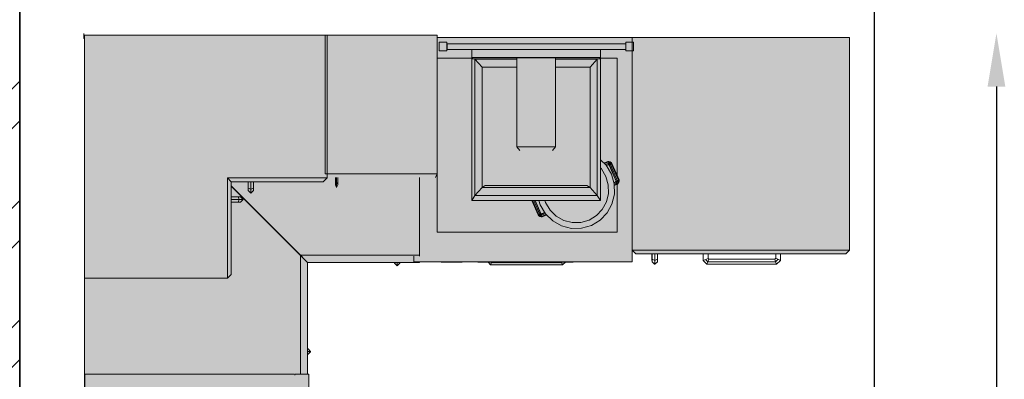
# Model space of a CAD drawing. Units: inches. Extents: x 3614 to 4242, y 2406 to 3033.
# Tile 5 of 10: x 3697 to 3808, y 2896 to 2936. Entities that reach past the tile are written whole.
import ezdxf

# ---------------------------------------------------------------- set-up
doc = ezdxf.new("R2010")
doc.units = ezdxf.units.IN
for name, color, linetype, lineweight in [('A-ANNO-DIMS', 2, 'Continuous', 18), ('A-FLOR-FIXT', 9, 'Continuous', 18), ('A-WALL', 7, 'Continuous', 35), ('A-WALL-PATT', 252, 'Continuous', 13)]:
    doc.layers.add(name, color=color, linetype=linetype, lineweight=lineweight)
doc.layers.add('hatch', color=254, linetype='Continuous')
doc.styles.get("Standard").update_dxf_attribs({"font": 'arial.ttf'})
doc.dimstyles.get("Standard").update_dxf_attribs({"dimtxt": 6, "dimasz": 6, "dimexe": 0.18, "dimexo": 0.0625, "dimgap": 0.09, "dimtad": 0, "dimtih": 1, "dimtoh": 1, "dimdec": 4, "dimzin": 0, "dimdsep": 46, "dimlunit": 4, "dimtxsty": 'Standard', "dimcen": 0.09, "dimse1": 1, "dimse2": 1, "dimadec": 0, "dimazin": 0, "dimtfac": 1, "dimtdec": 4, "dimtofl": 0, "dimtmove": 0, "dimatfit": 3, "dimfxl": 1, "dimtolj": 1, "dimtzin": 0, "dimarcsym": 0})

# ---------------------------------------------------------------- blocks, each defined once
blk = doc.blocks.new('kithen1')
at = {"layer": 'hatch'}
blk.add_hatch(color=256, dxfattribs=at).paths.add_polyline_path([(-2799.7, -8.3), (-2273.3, -8.3), (-2273.3, -1.7), (-2257.5, -1.7), (-2257.5, -1.1), (-1023.7, -1.1), (-1023.7, 0), (0, 0), (0, -0.3), (0.3, -0.3), (0.3, -1009.9), (-6.1, -1009.9), (-6.1, -2189.3), (-615.8, -2189.3), (-626.5, -2178.9), (-626.5, -1578.2), (-615.8, -1567.8), (-649.5, -1567.8), (-649.5, -1399.1), (-650.3, -1399.1), (-650.3, -1376.8), (-657.9, -1368.5), (-657.8, -1162.4), (-650.3, -1155.1), (-650.3, -1126.4), (-649.5, -1126.4), (-649.5, -1081.1), (-650.3, -1081.1), (-650.3, -1021.1), (-649.5, -1021.1), (-649.5, -959.1), (-651, -959.1), (-650.7, -903), (-653.5, -903), (-660.6, -895.5), (-660.5, -894.6), (-653.5, -887.1), (-651, -887.1), (-651, -638.7), (-651.2, -638.5), (-898.3, -638.5), (-898.3, -640.4), (-905.9, -647.4), (-906.8, -647.4), (-914.3, -640.4), (-914.3, -638.5), (-971.4, -638.5), (-971.4, -642.6), (-1016.2, -642.6), (-1016.2, -643.9), (-1023.8, -650.9), (-1024.7, -650.9), (-1032.2, -643.9), (-1032.2, -642.6), (-1179.7, -642.6), (-1188.8, -650.9), (-1395.6, -650.9), (-1403.7, -642.6), (-1813.5, -642.6), (-1822.6, -650.9), (-2029.4, -650.9), (-2037.5, -642.6), (-2257.5, -642.6), (-2257.5, -618.1), (-2261.3, -618.1), (-2271.7, -628.7), (-2458, -628.7), (-2727.7, -628.7), (-2727.7, -651.1), (-2735, -658.1), (-2735.9, -658), (-2743.2, -651.1), (-2743.2, -628.7), (-2789.4, -628.7), (-2799.7, -618.1)])
at = {"color": 0}
for p, q in [((0, 0), (-1023.7, 0)), ((-696.5, 0), (-696.5, -409.2)), ((-8.6, 1.9), (-10.5, 0)), ((-10.1, 0), (-8.2, 1.9)), ((-8.2, 1.9), (-8.3, 1.8)), ((-8.3, 1.9), (-8.3, 0)), ((5.4, 1.8), (-8.3, 1.8)), ((0, 0), (0, -694.7)), ((0, -0.3), (0, 0)), ((-2261.3, -8.3), (-2799.7, -8.3)), ((-2799.7, -8.3), (-2799.7, -618.1)), ((-2273.3, -1.9), (-2273.9, -1.9)), ((-2273.9, -1.9), (-2273.9, -8.3)), ((-2261.3, -1.7), (-2273.3, -1.7)), ((-2273.3, -1.7), (-2273.3, -8.3)), ((-2261.3, -601.6), (-2261.3, -1.7)), ((-2261.3, -618.1), (-2261.3, -8.3)), ((-2261, -8.5), (-2261.3, -8.5)), ((-971.4, -1.1), (-2257.5, -1.1)), ((-2257.5, -1.1), (-2257.5, -642.6)), ((-1023.7, -22.5), (-2210.1, -22.5)), ((-2210.1, -22.5), (-2210.1, -589.1)), ((-1023.7, -589.1), (-1023.7, -22.5)), ((-971.4, -1.1), (-971.4, -600.9)), ((0.3, -0.3), (0, -0.3)), ((0.3, -671.1), (0.3, -0.3)), ((-2257.5, -51.5), (-2261.3, -51.5)), ((-2261.3, -51.5), (-2261.3, -536.3)), ((-2183.7, -48.8), (-1056.9, -48.9)), ((-2169.4, -62.7), (-2183.7, -48.8)), ((-2183.7, -48.8), (-2183.7, -565)), ((-1056.9, -48.9), (-1071, -63.6)), ((-1056.9, -48.9), (-1056.9, -565)), ((-2169.7, -550.2), (-2169.4, -62.7)), ((-1071, -63.6), (-2169.4, -62.7)), ((-2103.6, -76.6), (-2136.6, -97.6)), ((-2135.1, -98.9), (-2102.3, -78.1)), ((-2100.1, -80.6), (-2132.5, -101.2)), ((-2057.7, -68.5), (-2103.6, -76.6)), ((-2102.3, -78.1), (-2056.8, -70)), ((-2100.1, -80.6), (-2102.3, -78.1)), ((-2055, -72.6), (-2100.1, -80.6)), ((-2093.2, -88.3), (-2100.1, -80.6)), ((-2049.7, -80.6), (-2093.2, -88.3)), ((-1740.9, -68.5), (-2057.7, -68.5)), ((-2056.8, -70), (-1741.9, -70)), ((-1743.7, -72.6), (-2055, -72.6)), ((-1749, -80.6), (-2049.7, -80.6)), ((-1716.2, -84.8), (-1749, -80.6)), ((-1709.7, -76.9), (-1743.7, -72.6)), ((-1741.9, -70), (-1707.6, -74.4)), ((-1706.4, -72.9), (-1740.9, -68.5)), ((-1678, -91.5), (-1709.7, -76.9)), ((-1707.6, -74.4), (-1675.5, -89.1)), ((-1674.1, -87.7), (-1706.4, -72.9)), ((-1071, -550.2), (-1071, -63.6)), ((-2136.6, -97.6), (-2156.1, -126.2)), ((-2154.5, -127.3), (-2135.1, -98.9)), ((-2132.5, -101.2), (-2151.7, -129.3)), ((-2124.5, -108.2), (-2143, -135.3)), ((-2132.5, -101.2), (-2135.1, -98.9)), ((-2124.5, -108.2), (-2132.5, -101.2)), ((-2093.2, -88.3), (-2124.5, -108.2)), ((-1685.6, -98.8), (-1716.2, -84.8)), ((-1678, -91.5), (-1685.6, -98.8)), ((-1685.6, -98.8), (-1660.4, -125.8)), ((-1651.9, -119.5), (-1678, -91.5)), ((-1675.5, -89.1), (-1649.1, -117.4)), ((-1647.6, -116.2), (-1674.1, -87.7)), ((-1523.7, -95.6), (-1554, -114.9)), ((-1481.5, -88.1), (-1523.7, -95.6)), ((-1523.7, -95.6), (-1509.8, -111.1)), ((-1189.8, -88.1), (-1481.5, -88.1)), ((-1416.2, -122.1), (-1396, -106.6)), ((-1396, -106.6), (-1372.5, -96.9)), ((-1372.5, -96.9), (-1347.3, -93.6)), ((-1347.3, -93.6), (-1322, -96.9)), ((-1322, -96.9), (-1298.5, -106.6)), ((-1298.5, -106.6), (-1278.3, -122.1)), ((-1283.4, -118.2), (-1268.1, -102.9)), ((-1268.1, -102.9), (-1230.5, -92.9)), ((-1230.5, -92.9), (-1193, -102.9)), ((-1193, -102.9), (-1165.5, -130.3)), ((-1157.9, -92.2), (-1189.8, -88.1)), ((-1128.2, -105.8), (-1157.9, -92.2)), ((-1143.5, -120.5), (-1128.2, -105.8)), ((-1128.2, -105.8), (-1103.8, -132)), ((-2156.1, -126.2), (-2163.3, -163.2)), ((-2161.7, -164.1), (-2154.5, -127.3)), ((-2151.7, -129.3), (-2158.8, -165.7)), ((-2151.7, -129.3), (-2154.5, -127.3)), ((-2143, -135.3), (-2151.7, -129.3)), ((-2149.9, -170.5), (-2143, -135.3)), ((-1660.4, -125.8), (-1651.9, -119.5)), ((-1648.8, -170.4), (-1660.4, -125.8)), ((-1649.1, -117.4), (-1651.9, -119.5)), ((-1651.9, -119.5), (-1639.9, -165.7)), ((-1649.1, -117.4), (-1637, -164.1)), ((-1635.3, -163.2), (-1647.6, -116.2)), ((-1554, -114.9), (-1572, -141.2)), ((-1431.7, -142.2), (-1416.2, -122.1)), ((-1278.3, -122.1), (-1262.8, -142.2)), ((-1252, -130.7), (-1263.1, -141.8)), ((-1249.5, -134.9), (-1261, -146.4)), ((-1246.6, -139.9), (-1258.4, -151.7)), ((-1252, -130.7), (-1230.5, -124.9)), ((-1249.5, -134.9), (-1230.5, -129.8)), ((-1230.5, -135.6), (-1246.6, -139.9)), ((-1246.6, -139.9), (-1244.8, -143)), ((-1244.8, -143), (-1230.5, -139.2)), ((-1230.5, -124.9), (-1209.1, -130.7)), ((-1230.5, -129.8), (-1211.6, -134.9)), ((-1214.5, -139.9), (-1230.5, -135.6)), ((-1230.5, -135.6), (-1230.5, -139.2)), ((-1230.5, -139.2), (-1216.3, -143)), ((-1216.3, -143), (-1214.5, -139.9)), ((-1211.6, -134.9), (-1214.5, -139.9)), ((-1214.5, -139.9), (-1202.7, -151.7)), ((-1211.6, -134.9), (-1197.7, -148.8)), ((-1209.1, -130.7), (-1193.4, -146.3)), ((-1165.5, -130.3), (-1155.5, -167.7)), ((-1103.8, -132), (-1120.8, -144.8)), ((-1103.8, -132), (-1092.5, -175.3)), ((-2163.3, -163.2), (-2163.3, -447.5)), ((-2161.7, -446.6), (-2161.7, -164.1)), ((-2158.8, -165.7), (-2158.8, -445)), ((-1639.9, -165.7), (-1639.9, -445)), ((-1637, -164.1), (-1637, -446.6)), ((-1635.3, -447.4), (-1635.3, -163.2)), ((-1572, -141.2), (-1578.6, -175.3)), ((-1572, -141.2), (-1554.6, -153.3)), ((-1444.8, -190.8), (-1441.5, -165.7)), ((-1441.5, -165.7), (-1431.7, -142.2)), ((-1262.8, -142.2), (-1253, -165.7)), ((-1258.4, -151.7), (-1258.6, -152.3)), ((-1255.2, -153.5), (-1258.4, -151.7)), ((-1255.2, -153.5), (-1256.4, -157.6)), ((-1244.8, -143), (-1255.2, -153.5)), ((-1253, -165.7), (-1249.7, -190.8)), ((-1205.8, -153.5), (-1216.3, -143)), ((-1202.7, -151.7), (-1205.8, -153.5)), ((-1205.8, -153.5), (-1202, -167.7)), ((-1202, -167.7), (-1205.8, -181.9)), ((-1198.4, -167.7), (-1202.7, -151.7)), ((-1202.7, -183.7), (-1198.4, -167.7)), ((-1202, -167.7), (-1198.4, -167.7)), ((-1197.7, -148.8), (-1192.6, -167.7)), ((-1192.6, -167.7), (-1197.7, -186.6)), ((-1193.4, -146.3), (-1187.6, -167.7)), ((-1187.6, -167.7), (-1193.4, -189.1)), ((-1155.5, -167.7), (-1165.5, -205.1)), ((-2149.9, -440.2), (-2149.9, -170.5)), ((-1648.8, -440.2), (-1648.8, -170.4)), ((-1578.6, -175.3), (-1578.6, -437)), ((-1441.5, -216), (-1444.8, -190.8)), ((-1249.7, -190.8), (-1253, -216)), ((-1250.2, -186.9), (-1244.8, -192.3)), ((-1246.6, -195.5), (-1249.9, -192.2)), ((-1244.8, -192.3), (-1246.6, -195.5)), ((-1230.5, -199.7), (-1246.6, -195.5)), ((-1230.5, -196.1), (-1244.8, -192.3)), ((-1216.3, -192.3), (-1230.5, -196.1)), ((-1214.5, -195.5), (-1230.5, -199.7)), ((-1230.5, -196.1), (-1230.5, -199.7)), ((-1205.8, -181.9), (-1216.3, -192.3)), ((-1216.3, -192.3), (-1214.5, -195.5)), ((-1214.5, -195.5), (-1202.7, -183.7)), ((-1211.6, -200.5), (-1214.5, -195.5)), ((-1197.7, -186.6), (-1211.6, -200.5)), ((-1193.4, -189.1), (-1209.1, -204.7)), ((-1205.8, -181.9), (-1202.7, -183.7)), ((-1092.5, -175.3), (-1092.5, -437)), ((-1442, -212), (-1442.1, -213.6)), ((-1442.1, -213.6), (-1441.9, -216.3)), ((-1441.9, -216.3), (-1441.5, -218.2)), ((-1431.7, -239.4), (-1441.5, -216)), ((-1441.5, -218.2), (-1440.8, -218.9)), ((-1440.8, -218.9), (-1440.3, -218.9)), ((-1253, -216), (-1262.8, -239.4)), ((-1230.5, -210.4), (-1251.6, -204.8)), ((-1250.8, -199.1), (-1249.5, -200.5)), ((-1211.6, -200.5), (-1230.5, -205.5)), ((-1209.1, -204.7), (-1230.5, -210.4)), ((-1165.5, -205.1), (-1193, -232.5)), ((-1416.2, -259.6), (-1431.7, -239.4)), ((-1262.8, -239.4), (-1278.3, -259.6)), ((-1230.5, -242.5), (-1260.7, -234.4)), ((-1193, -232.5), (-1230.5, -242.5)), ((-1914.6, -272.1), (-1926.9, -292)), ((-1891.8, -266.6), (-1914.6, -272.1)), ((-1871.8, -278.8), (-1891.8, -266.6)), ((-1866.3, -301.6), (-1871.8, -278.8)), ((-1396, -275), (-1416.2, -259.6)), ((-1372.5, -284.8), (-1396, -275)), ((-1298.5, -275), (-1322, -284.8)), ((-1278.3, -259.6), (-1298.5, -275)), ((-1926.9, -292), (-1921.4, -314.8)), ((-1878.5, -321.5), (-1866.3, -301.6)), ((-1526.8, -324.6), (-1493.1, -302.1)), ((-1493.1, -302.2), (-1526.8, -324.6)), ((-1492.2, -304.2), (-1525.2, -326.2)), ((-1493.1, -302.1), (-1453.2, -294.2)), ((-1453.2, -294.3), (-1493.1, -302.2)), ((-1453.2, -296.5), (-1492.2, -304.2)), ((-1453.2, -294.2), (-1413.4, -302.1)), ((-1413.4, -302.2), (-1453.2, -294.3)), ((-1453.2, -294.3), (-1453.2, -296.5)), ((-1453.2, -296.5), (-1414.2, -304.2)), ((-1413.4, -302.1), (-1379.6, -324.6)), ((-1379.6, -324.6), (-1413.4, -302.2)), ((-1347.3, -288.1), (-1372.5, -284.8)), ((-1364, -321.4), (-1354.5, -287.1)), ((-1322, -284.8), (-1347.3, -288.1)), ((-1316.5, -282.5), (-1307.2, -290.8)), ((-1307.2, -290.8), (-1307.2, -321.4)), ((-1921.4, -314.8), (-1901.4, -327)), ((-1901.4, -327), (-1878.5, -321.5)), ((-1526.8, -324.6), (-1549.4, -358.3)), ((-1549.4, -358.3), (-1526.8, -324.6)), ((-1525.2, -326.2), (-1547.3, -359.2)), ((-1514.5, -337), (-1533.3, -365)), ((-1486.4, -318.2), (-1514.5, -337)), ((-1453.2, -311.7), (-1486.4, -318.2)), ((-1453.2, -311.7), (-1420.1, -318.2)), ((-1453.2, -338.2), (-1453.2, -311.7)), ((-1420.1, -318.2), (-1392, -337)), ((-1392, -337), (-1373.2, -365)), ((-1379.6, -324.6), (-1357, -358.3)), ((-1357, -358.3), (-1379.6, -324.6)), ((-1363.6, -324.3), (-1364, -321.4)), ((-1361.6, -328), (-1363.6, -324.3)), ((-1357.9, -330.6), (-1361.6, -328)), ((-1352.7, -331.6), (-1357.9, -330.6)), ((-1318.5, -331.6), (-1352.7, -331.6)), ((-1314.3, -331), (-1318.5, -331.6)), ((-1310.7, -329.1), (-1314.3, -331)), ((-1308.2, -326), (-1310.7, -329.1)), ((-1307.2, -321.4), (-1308.2, -326)), ((-1248.3, -343.1), (-1240.7, -330.6)), ((-1243.2, -344.9), (-1236.8, -334.2)), ((-1240.7, -330.6), (-1228.9, -321.9)), ((-1227.6, -324.8), (-1238.3, -332.8)), ((-1236.8, -334.2), (-1226.7, -326.8)), ((-1228.9, -321.9), (-1214.7, -318.4)), ((-1227.6, -324.8), (-1228.3, -323.3)), ((-1214.6, -321.6), (-1227.6, -324.8)), ((-1226.7, -326.8), (-1214.5, -323.7)), ((-1214.7, -318.4), (-1200.3, -320.6)), ((-1214.7, -319.9), (-1214.6, -321.6)), ((-1214.6, -321.6), (-1201.4, -323.6)), ((-1214.5, -323.7), (-1202.1, -325.6)), ((-1202.1, -325.6), (-1191.3, -332)), ((-1201.4, -323.6), (-1200.8, -322)), ((-1201.4, -323.6), (-1189.9, -330.5)), ((-1200.3, -320.6), (-1187.7, -328.1)), ((-1191.3, -332), (-1183.9, -342.1)), ((-1189.9, -330.5), (-1188.7, -329.2)), ((-1189.9, -330.5), (-1181.9, -341.2)), ((-1187.7, -328.1), (-1179, -339.8)), ((-1549.4, -358.3), (-1557.3, -398)), ((-1557.3, -398), (-1549.4, -358.3)), ((-1547.3, -359.2), (-1555.1, -398)), ((-1533.3, -365), (-1539.9, -398)), ((-1508.7, -375.1), (-1495.7, -355.7)), ((-1495.7, -355.7), (-1476.2, -342.8)), ((-1476.2, -342.8), (-1453.2, -338.2)), ((-1430.3, -342.8), (-1453.2, -338.2)), ((-1410.8, -355.7), (-1430.3, -342.8)), ((-1397.8, -375.1), (-1410.8, -355.7)), ((-1373.2, -365), (-1366.6, -398)), ((-1357, -358.3), (-1349.1, -398)), ((-1349.1, -398), (-1357, -358.3)), ((-1250.4, -357.6), (-1248.3, -343.1)), ((-1246.9, -371.7), (-1250.4, -357.6)), ((-1245.1, -357.3), (-1243.2, -344.9)), ((-1242, -369.4), (-1245.1, -357.3)), ((-1183.9, -342.1), (-1180.8, -354.2)), ((-1180.8, -354.2), (-1182.7, -366.6)), ((-1181.9, -341.2), (-1180.4, -340.5)), ((-1181.9, -341.2), (-1178.7, -354.1)), ((-1178.7, -354.1), (-1180.7, -367.3)), ((-1179, -339.8), (-1175.5, -354)), ((-1178.7, -354.1), (-1177, -354.1)), ((-1175.5, -354), (-1177.6, -368.4)), ((-1513.2, -398), (-1508.7, -375.1)), ((-1393.2, -398), (-1397.8, -375.1)), ((-1238.2, -383.5), (-1246.9, -371.7)), ((-1234.6, -379.5), (-1242, -369.4)), ((-1225.6, -391), (-1238.2, -383.5)), ((-1223.8, -385.9), (-1234.6, -379.5)), ((-1211.2, -393.1), (-1225.6, -391)), ((-1211.4, -387.8), (-1223.8, -385.9)), ((-1199.2, -384.8), (-1211.4, -387.8)), ((-1197, -389.6), (-1211.2, -393.1)), ((-1202.1, -390.9), (-1202.4, -391)), ((-1202.4, -391), (-1202, -390.9)), ((-1202.4, -391), (-1202.4, -391)), ((-1202.4, -391), (-1202.3, -391.3)), ((-1202.3, -391.3), (-1200.2, -395.7)), ((-1202, -390.9), (-1202.1, -390.9)), ((-1201.7, -390.8), (-1199.7, -395.1)), ((-1199.7, -395.1), (-1198, -394.1)), ((-1189.2, -377.3), (-1199.2, -384.8)), ((-1187.6, -378.8), (-1198.3, -386.7)), ((-1185.2, -380.9), (-1197, -389.6)), ((-1193.3, -386.9), (-1194.2, -387.6)), ((-1193.1, -386.7), (-1193.3, -386.9)), ((-1193.3, -386.9), (-1191.3, -391.2)), ((-1191.3, -391.2), (-1193.2, -391.8)), ((-1192.7, -386.5), (-1192.9, -386.6)), ((-1192.6, -386.8), (-1192.7, -386.5)), ((-1190.5, -391.2), (-1192.6, -386.8)), ((-1191.3, -391.2), (-1190.5, -391.2)), ((-1188.3, -397.5), (-1191.3, -391.2)), ((-1190.5, -391.2), (-1187.6, -397.2)), ((-1182.7, -366.6), (-1189.2, -377.3)), ((-1180.7, -367.3), (-1187.6, -378.8)), ((-1187.6, -378.8), (-1186.3, -379.9)), ((-1177.6, -368.4), (-1185.2, -380.9)), ((-1180.7, -367.3), (-1179.1, -367.9)), ((-1557.3, -398), (-1549.4, -437.8)), ((-1549.4, -437.8), (-1557.3, -398)), ((-1555.1, -398), (-1547.3, -436.9)), ((-1539.9, -398), (-1533.3, -431.1)), ((-1508.7, -420.9), (-1513.2, -398)), ((-1495.7, -440.4), (-1508.7, -420.9)), ((-1410.8, -440.4), (-1397.8, -420.9)), ((-1397.8, -420.9), (-1393.2, -398)), ((-1366.6, -398), (-1373.2, -431.1)), ((-1349.1, -398), (-1357, -437.8)), ((-1357, -437.8), (-1349.1, -398)), ((-1200.2, -395.7), (-1199.7, -395.1)), ((-1200.2, -395.7), (-1197.3, -401.8)), ((-1199.7, -395.1), (-1196.7, -401.5)), ((-1197.3, -401.8), (-1196.7, -401.5)), ((-1197.3, -401.8), (-1194.5, -407.8)), ((-1196.7, -401.5), (-1190.1, -398.4)), ((-1196.7, -401.5), (-1193.7, -407.8)), ((-1194.5, -407.8), (-1193.7, -407.8)), ((-1192.4, -412.2), (-1194.5, -407.8)), ((-1193.7, -407.8), (-1191.8, -407.2)), ((-1193.7, -407.8), (-1191.5, -412.5)), ((-1191.6, -413.9), (-1192.4, -412.2)), ((-1190.7, -414.2), (-1191.6, -413.9)), ((-1188.7, -413.8), (-1190.7, -414.2)), ((-1190.1, -398.4), (-1188.3, -397.5)), ((-1186.2, -412.8), (-1188.7, -413.8)), ((-1187.6, -397.2), (-1188.3, -397.5)), ((-1188.3, -397.5), (-1185.3, -403.9)), ((-1184.8, -403.3), (-1187.6, -397.2)), ((-1185.3, -403.9), (-1186.9, -404.9)), ((-1183.8, -411.5), (-1186.2, -412.8)), ((-1185.3, -403.9), (-1184.8, -403.3)), ((-1183.1, -408.5), (-1185.3, -403.9)), ((-1184.8, -403.3), (-1182.7, -407.7)), ((-1182.3, -410.2), (-1183.8, -411.5)), ((-1182.7, -407.7), (-1181.9, -409.3)), ((-1181.9, -409.3), (-1182.3, -410.2)), ((-696.5, -409.2), (-408.8, -409.2)), ((-685.5, -420.3), (-696.5, -409.2)), ((-419.9, -420.3), (-685.5, -420.3)), ((-432.1, -420.3), (-630.9, -618.1)), ((-630.6, -618.4), (-431.9, -420.3)), ((-614.8, -602.2), (-432.2, -420.3)), ((-431.9, -420.3), (-614.5, -602.5)), ((-432, -420.3), (-607.9, -595.8)), ((-432.1, -420.3), (-607.9, -595.4)), ((-478.5, -420.3), (-478.5, -439.9)), ((-470.7, -443), (-470.7, -420.3)), ((-462.9, -420.3), (-462.9, -439.9)), ((-408.8, -409.2), (-419.9, -420.3)), ((-419.9, -683.7), (-419.9, -420.3)), ((-408.8, -409.2), (-408.8, -694.7)), ((-2163.3, -447.5), (-2159.9, -473.6)), ((-2158.2, -472.6), (-2161.7, -446.6)), ((-2158.8, -445), (-2155.4, -470.7)), ((-2146.6, -465), (-2149.9, -440.2)), ((-1658, -480.4), (-1648.8, -440.2)), ((-1639.9, -445), (-1649.4, -486.6)), ((-1637, -446.6), (-1646.6, -488.6)), ((-1645, -489.8), (-1635.3, -447.4)), ((-1578.6, -437), (-1575.5, -461.1)), ((-1575.5, -461.1), (-1557.8, -449.7)), ((-1549.4, -437.8), (-1526.8, -471.4)), ((-1526.8, -471.4), (-1549.4, -437.8)), ((-1547.3, -436.9), (-1525.2, -469.8)), ((-1533.3, -431.1), (-1514.5, -459.1)), ((-1476.2, -453.3), (-1495.7, -440.4)), ((-1430.3, -453.3), (-1410.8, -440.4)), ((-1373.2, -431.1), (-1392, -459.1)), ((-1357, -437.8), (-1379.6, -471.4)), ((-1379.6, -471.4), (-1357, -437.8)), ((-1092.5, -437), (-1101.4, -476)), ((-478.5, -439.9), (-470.7, -443)), ((-478.5, -439.9), (-478.5, -446.8)), ((-478.5, -446.8), (-470.7, -454.1)), ((-462.9, -439.9), (-470.7, -443)), ((-470.7, -443), (-470.7, -454.1)), ((-470.7, -454.1), (-462.9, -446.8)), ((-462.9, -446.8), (-462.9, -439.9)), ((-2159.9, -473.6), (-2141.1, -508.3)), ((-2139.6, -507.1), (-2158.2, -472.6)), ((-2155.4, -470.7), (-2146.6, -465)), ((-2137, -504.8), (-2155.4, -470.7)), ((-2146.6, -465), (-2128.8, -498)), ((-1575.5, -461.1), (-1558.2, -493)), ((-1493.1, -493.9), (-1526.8, -471.4)), ((-1526.8, -471.4), (-1493.1, -493.9)), ((-1525.2, -469.8), (-1492.2, -491.9)), ((-1514.5, -459.1), (-1486.4, -477.9)), ((-1486.4, -477.9), (-1453.2, -484.4)), ((-1453.2, -457.9), (-1476.2, -453.3)), ((-1453.2, -457.9), (-1430.3, -453.3)), ((-1453.2, -484.4), (-1453.2, -457.9)), ((-1420.1, -477.9), (-1453.2, -484.4)), ((-1392, -459.1), (-1420.1, -477.9)), ((-1379.6, -471.4), (-1413.4, -493.9)), ((-1413.4, -493.9), (-1379.6, -471.4)), ((-1101.4, -476), (-1123, -502.7)), ((-1101.4, -476), (-1118.7, -463.5)), ((-444.9, -468.4), (-452.2, -476.2)), ((-452.2, -476.2), (-441.1, -476.2)), ((-452.2, -476.2), (-444.9, -484)), ((-419.9, -468.4), (-444.9, -468.4)), ((-441.1, -476.2), (-438, -468.4)), ((-419.9, -476.2), (-441.1, -476.2)), ((-441.1, -476.2), (-438, -484)), ((-2137, -504.8), (-2139.6, -507.1)), ((-2105.6, -531.3), (-2139.6, -507.1)), ((-2128.8, -498), (-2137, -504.8)), ((-2103.3, -528.8), (-2137, -504.8)), ((-2128.8, -498), (-2096.3, -521.1)), ((-2085.5, -509.3), (-2116.3, -487.4)), ((-2060.9, -482.3), (-2085.5, -509.3)), ((-1680.2, -507.9), (-1658, -480.4)), ((-1649.4, -486.6), (-1672.5, -515.1)), ((-1646.6, -488.6), (-1669.9, -517.4)), ((-1668.5, -518.8), (-1645, -489.8)), ((-1649.4, -486.6), (-1658, -480.4)), ((-1646.6, -488.6), (-1649.4, -486.6)), ((-1558.2, -493), (-1526.7, -515.5)), ((-1526.7, -515.5), (-1512.6, -500.1)), ((-1453.2, -501.8), (-1493.1, -493.9)), ((-1493.1, -493.9), (-1453.2, -501.8)), ((-1492.2, -491.9), (-1453.2, -499.6)), ((-1453.2, -499.6), (-1414.2, -491.9)), ((-1413.4, -493.9), (-1453.2, -501.8)), ((-1453.2, -501.8), (-1413.4, -493.9)), ((-1453.2, -499.6), (-1453.2, -501.8)), ((-1123, -502.7), (-1153.4, -518.8)), ((-1123, -502.7), (-1138.7, -488.2)), ((-444.9, -484), (-438, -484)), ((-438, -484), (-419.9, -484)), ((-2257.5, -535.3), (-2257.9, -535.3)), ((-2141.1, -508.3), (-2106.9, -532.7)), ((-2106.9, -532.7), (-2057.7, -542.2)), ((-2103.3, -528.8), (-2105.6, -531.3)), ((-2056.8, -540.7), (-2105.6, -531.3)), ((-2096.3, -521.1), (-2103.3, -528.8)), ((-2055, -538.1), (-2103.3, -528.8)), ((-2096.3, -521.1), (-2085.5, -509.3)), ((-2049.7, -530.1), (-2096.3, -521.1)), ((-2085.5, -509.3), (-2041.5, -517.8)), ((-1749, -530.1), (-2049.7, -530.1)), ((-1749, -530.1), (-1797.1, -530.1)), ((-1711.5, -524.5), (-1749, -530.1)), ((-1704.9, -532.3), (-1743.7, -538.1)), ((-1741.9, -540.7), (-1702.7, -534.9)), ((-1680.2, -507.9), (-1711.5, -524.5)), ((-1672.5, -515.1), (-1704.9, -532.3)), ((-1702.7, -534.9), (-1669.9, -517.4)), ((-1668.5, -518.8), (-1701.5, -536.3)), ((-1672.5, -515.1), (-1680.2, -507.9)), ((-1669.9, -517.4), (-1672.5, -515.1)), ((-1189.8, -524.2), (-1668.5, -518.8)), ((-1481.5, -524.2), (-1668.5, -518.8)), ((-1526.7, -515.5), (-1481.5, -524.2)), ((-1189.8, -524.2), (-1481.5, -524.2)), ((-1153.4, -518.8), (-1189.8, -524.2)), ((-540.1, -527.9), (-540.1, -528.1)), ((-2183.7, -565), (-2169.7, -550.2)), ((-1793.1, -550.2), (-2169.7, -550.2)), ((-2057.7, -542.2), (-2056.8, -540.7)), ((-1783.5, -542.2), (-2057.7, -542.2)), ((-1781.7, -540.7), (-2056.8, -540.7)), ((-1778.6, -538.1), (-2055, -538.1)), ((-1743.7, -538.1), (-1797.1, -538.1)), ((-1741.9, -540.7), (-1797.1, -540.7)), ((-1740.9, -542.2), (-1797.1, -542.2)), ((-1071, -550.2), (-1797.1, -550.2)), ((-1740.9, -542.2), (-1741.9, -540.7)), ((-1701.5, -536.3), (-1740.9, -542.2)), ((-1056.9, -565), (-1071, -550.2)), ((-2210.1, -589.1), (-1789.4, -589.1)), ((-1797.1, -565), (-2183.7, -565)), ((-1056.9, -565), (-1797.1, -565)), ((-1797.1, -589.1), (-1023.7, -589.1)), ((-597, -584.5), (-597, -584.9)), ((-2799.7, -618.1), (-2261.3, -618.1)), ((-2789.4, -628.7), (-2799.7, -618.1)), ((-2261.3, -618.1), (-2271.7, -628.7)), ((-2261, -596.4), (-2261.3, -596.4)), ((-2261.3, -626.3), (-2261.3, -601.6)), ((-972.7, -601.6), (-972.7, -603)), ((-971.4, -600.6), (-971.4, -601.6)), ((-971.4, -603), (-971.4, -642.6)), ((-630.9, -618.1), (-971.4, -618.1)), ((-611.6, -599.1), (-651.2, -638.5)), ((-611.6, -599.4), (-651, -638.7)), ((-642.6, -629.8), (-630.9, -618.1)), ((-630.6, -618.4), (-642.3, -630.1)), ((-630.9, -618.1), (-614.8, -602.2)), ((-614.5, -602.5), (-630.6, -618.4)), ((-630.6, -959.1), (-630.6, -618.4)), ((-620.1, -607.7), (-609.4, -597.1)), ((-619.9, -607.6), (-620.1, -607.6)), ((-620.1, -607.9), (-620.1, -607.7)), ((-609, -596.9), (-609.4, -596.9)), ((-609.4, -597.1), (-609.4, -597.2)), ((-607.9, -595.4), (-607.9, -595.8)), ((-2271.7, -628.7), (-2789.4, -628.7)), ((-2743.2, -628.7), (-2743.2, -644.8)), ((-2743.2, -644.8), (-2742.3, -644.5)), ((-2743.2, -651.1), (-2743.2, -644.8)), ((-2742.3, -628.7), (-2742.3, -644.4)), ((-2742.3, -644.4), (-2734.9, -647.4)), ((-2742.3, -644.4), (-2742.3, -651.1)), ((-2734.9, -647.4), (-2735, -658.1)), ((-2734.9, -647.4), (-2734.9, -628.7)), ((-2727.7, -644.4), (-2734.9, -647.4)), ((-2727.7, -628.7), (-2727.7, -644.4)), ((-2727.7, -651.1), (-2727.7, -644.4)), ((-2679.7, -628.7), (-2679.4, -647.7)), ((-2679.4, -647.7), (-2665.9, -642)), ((-2669.5, -658), (-2679.4, -647.7)), ((-2666.7, -651.1), (-2672.6, -644.8)), ((-2663.9, -644.2), (-2666.7, -651.1)), ((-2665.6, -628.7), (-2665.9, -642)), ((-2665.9, -642), (-2663.9, -644.2)), ((-2663.9, -644.2), (-2474.9, -644.1)), ((-2474.9, -644.1), (-2471.7, -641.3)), ((-2474.9, -644.1), (-2472.3, -651.1)), ((-2472.3, -651.1), (-2465, -644.4)), ((-2471.7, -641.3), (-2472, -628.7)), ((-2458.4, -647.4), (-2471.7, -641.3)), ((-2458.4, -647.4), (-2469.7, -658.1)), ((-2458, -628.7), (-2458.4, -647.4)), ((-2261.3, -643.6), (-2261.3, -626.3)), ((-2257.5, -642.6), (-1797.1, -642.6)), ((-2037.5, -642.6), (-2029.4, -650.9)), ((-2029.4, -650.9), (-2026.5, -643.9)), ((-2026.5, -643.9), (-2027.8, -642.6)), ((-2025.9, -642.6), (-2026.5, -643.9)), ((-2026.5, -643.9), (-1828.9, -643.9)), ((-1825.3, -643.9), (-1828.9, -643.9)), ((-1825.8, -642.6), (-1825.3, -643.9)), ((-1825.3, -643.9), (-1823.8, -642.6)), ((-1822.6, -650.9), (-1825.3, -643.9)), ((-1813.5, -642.6), (-1822.6, -650.9)), ((-971.4, -642.6), (-1797.1, -642.6)), ((-1395.6, -650.9), (-1403.7, -642.6)), ((-1392.7, -643.9), (-1395.6, -650.9)), ((-1394, -642.6), (-1392.7, -643.9)), ((-1392.7, -643.9), (-1392.1, -642.6)), ((-1191.5, -643.9), (-1392.7, -643.9)), ((-1192, -642.6), (-1191.5, -643.9)), ((-1191.5, -643.9), (-1190, -642.6)), ((-1188.8, -650.9), (-1191.5, -643.9)), ((-1179.7, -642.6), (-1188.8, -650.9)), ((-1032.2, -643.9), (-1032.2, -642.6)), ((-1031.4, -643.1), (-1032.2, -643.9)), ((-1031.4, -643.9), (-1032.2, -643.9)), ((-1032.2, -643.9), (-1024.7, -650.9)), ((-1031.4, -642.6), (-1031.4, -643.9)), ((-1023.8, -650.9), (-1031.4, -643.9)), ((-1023.8, -650.9), (-1023.8, -642.6)), ((-1016.2, -643.9), (-1023.8, -650.9)), ((-1016.2, -642.6), (-1016.2, -643.9)), ((-971.4, -635.7), (-971.4, -641.8)), ((-971.4, -641.8), (-971.4, -638.3)), ((-651.2, -638.5), (-971.4, -638.5)), ((-914.3, -640.4), (-914.4, -638.5)), ((-913.5, -639.6), (-914.3, -640.4)), ((-913.5, -640.4), (-914.3, -640.4)), ((-914.3, -640.4), (-906.8, -647.3)), ((-913.5, -638.5), (-913.5, -640.4)), ((-905.9, -647.4), (-913.5, -640.4)), ((-906.8, -647.3), (-905.9, -647.4)), ((-905.9, -647.4), (-905.9, -638.5)), ((-898.3, -640.4), (-905.9, -647.4)), ((-898.3, -638.5), (-898.3, -640.4)), ((-651, -638.7), (-651, -959.1)), ((-2742.3, -650.3), (-2743.2, -651.1)), ((-2742.3, -651.1), (-2743.2, -651.1)), ((-2743.2, -651.1), (-2735.9, -658)), ((-2735, -658.1), (-2742.3, -651.1)), ((-2735.9, -658), (-2735, -658.1)), ((-2735, -658.1), (-2727.7, -651.1)), ((-2666.7, -651.1), (-2669.5, -658)), ((-2669.5, -658), (-2469.7, -658.1)), ((-2472.3, -651.1), (-2666.7, -651.1)), ((-2469.7, -658.1), (-2472.3, -651.1)), ((-2029.4, -650.9), (-1828.9, -650.9)), ((-1822.6, -650.9), (-1828.9, -650.9)), ((-1395.6, -650.9), (-1188.8, -650.9)), ((-1024.7, -650.9), (-1023.8, -650.9)), ((0, -694.7), (0, -671.1)), ((0, -671.1), (0.3, -671.1)), ((-408.8, -694.7), (-419.9, -683.7)), ((0, -694.7), (-408.8, -694.7)), ((-0.1, -689.2), (-397.2, -689.2)), ((-397.2, -689.2), (-397.2, -1009.9)), ((-0.1, -1009.9), (-0.1, -689.2)), ((-0.1, -699.8), (-0.1, -998.7)), ((0.3, -700.4), (-0.1, -700.4)), ((0.3, -998.7), (0.3, -700.4)), ((-429, -718.2), (-436, -721.9)), ((-436, -721.9), (-425.3, -721.9)), ((-436, -721.9), (-429, -725.7)), ((-407.9, -718.2), (-429, -718.2)), ((-429, -725.7), (-422.2, -725.7)), ((-425.3, -721.9), (-422.2, -718.2)), ((-407.9, -721.9), (-425.3, -721.9)), ((-425.3, -721.9), (-422.2, -725.7)), ((-422.2, -725.7), (-407.9, -725.7)), ((-653.5, -887.9), (-660.6, -895.5)), ((-660.6, -895.5), (-660.5, -894.6)), ((-660.6, -895.5), (-651, -895.5)), ((-653.5, -903), (-660.6, -895.5)), ((-660.5, -894.6), (-653.5, -887.1)), ((-651, -887), (-653.5, -887.1)), ((-653.5, -887.1), (-652.7, -887.9)), ((-653.5, -887.1), (-653.5, -887.9)), ((-653.5, -887.9), (-651, -887.9)), ((-651, -903), (-653.5, -903)), ((-633.4, -942.7), (-649.5, -942.7)), ((-649.5, -942.7), (-649.5, -1567.8)), ((-651, -959.1), (-649.5, -959.1)), ((-630.6, -959.1), (-633.4, -959.1)), ((-407.9, -959.1), (-630.6, -959.1)), ((-398.5, -1009.2), (-564.1, -1009.2)), ((-564.1, -1009.2), (-564.1, -1525)), ((-397.2, -1009.9), (-407.9, -1004.5)), ((-397.2, -1009.9), (-0.1, -1009.9)), ((-65.6, -1009.9), (-65.6, -1108.4)), ((-6.1, -1009.9), (-6.1, -1567.8)), ((-0.1, -998.7), (0.3, -998.7)), ((-649.5, -1021.1), (-650.3, -1021.1)), ((-650.3, -1021.1), (-650.3, -1081.1)), ((-20.3, -1015.5), (-44.8, -1015.5)), ((-44.8, -1015.5), (-44.8, -1037.5)), ((-44.8, -1037.5), (-20.3, -1037.5)), ((-24.8, -1038), (-40.6, -1038)), ((-40.6, -1038), (-40.6, -1549.4)), ((-24.8, -1549.4), (-24.8, -1038)), ((-20.3, -1037.5), (-20.3, -1015.5)), ((-650.3, -1081.1), (-649.5, -1081.1)), ((-649.5, -1126.4), (-650.3, -1126.4)), ((-650.3, -1126.4), (-650.3, -1186.4)), ((-62.5, -1108.4), (-473.1, -1108.4)), ((-473.1, -1108.4), (-459.2, -1117.2)), ((-473.1, -1108.4), (-473.1, -1476.7)), ((-459.2, -1117.2), (-68.2, -1117.2)), ((-459.2, -1467.9), (-459.2, -1117.2)), ((-459.2, -1117.2), (-435.9, -1138.2)), ((-91.6, -1138.2), (-68.2, -1117.2)), ((-68.2, -1117.2), (-67.2, -1115.5)), ((-68.2, -1117.2), (-68.2, -1237.1)), ((-64.1, -1108.4), (-67.2, -1111.2)), ((-67.2, -1111.2), (-67.2, -1237.1)), ((-40.9, -1108.4), (-64.1, -1108.4)), ((-64.1, -1108.4), (-64.1, -1476.7)), ((-40.9, -1476.7), (-40.9, -1108.4)), ((-650.3, -1155.1), (-657.8, -1162.4)), ((-435.9, -1138.2), (-91.6, -1138.2)), ((-435.9, -1138.2), (-430.1, -1147)), ((-435.9, -1447), (-435.9, -1138.2)), ((-430.1, -1147), (-430.1, -1438.2)), ((-91.6, -1138.2), (-91.6, -1237.1)), ((-657.8, -1162.4), (-657.9, -1368.5)), ((-657.8, -1162.4), (-650.8, -1165.4)), ((-650.8, -1165.4), (-650.3, -1164.8)), ((-650.8, -1365.8), (-650.8, -1165.4)), ((-650.8, -1165.4), (-650.3, -1165.6)), ((-650.3, -1186.4), (-649.5, -1186.4)), ((-649.5, -1231.7), (-650.3, -1231.7)), ((-650.3, -1231.7), (-650.3, -1291.7)), ((-320.2, -1237.1), (-330.5, -1246.3)), ((-64.3, -1237.1), (-320.2, -1237.1)), ((-320.2, -1237.1), (-320.2, -1348.4)), ((-64.3, -1348.4), (-64.3, -1237.1)), ((-650.3, -1291.7), (-649.5, -1291.7)), ((-473.1, -1280.2), (-515, -1298.2)), ((-473.1, -1282.1), (-514, -1299.7)), ((-473.1, -1286.3), (-512, -1302.3)), ((-473.1, -1289.8), (-511.2, -1305.5)), ((-473.1, -1290.3), (-510.4, -1305.8)), ((-511.4, -1319.5), (-531.9, -1340.4)), ((-519.1, -1303.5), (-520.1, -1306.8)), ((-520.1, -1306.8), (-520.1, -1310.2)), ((-520.1, -1310.2), (-514.9, -1323)), ((-517.4, -1300.6), (-519.1, -1303.5)), ((-517.7, -1304.5), (-518.6, -1307.4)), ((-518.6, -1307.4), (-518.6, -1310.5)), ((-518.6, -1310.5), (-513.9, -1322)), ((-516.2, -1301.9), (-517.7, -1304.5)), ((-515.4, -1308), (-517.7, -1304.5)), ((-515, -1298.2), (-517.4, -1300.6)), ((-514, -1299.7), (-516.2, -1301.9)), ((-515.4, -1308), (-516.2, -1301.9)), ((-514, -1299.7), (-515.4, -1308)), ((-512, -1302.3), (-515.4, -1308)), ((-515.4, -1308), (-512.4, -1308.2)), ((-511.2, -1319.3), (-515.4, -1308)), ((-512, -1302.3), (-514, -1299.7)), ((-511.2, -1305.5), (-512.4, -1308.2)), ((-512.4, -1308.2), (-511.3, -1307.8)), ((-512.4, -1308.2), (-508, -1317.5)), ((-512.4, -1308.2), (-508.5, -1317.7)), ((-508.7, -1317.8), (-512.4, -1308.2)), ((-511.2, -1305.5), (-512, -1302.3)), ((-486.2, -1304.5), (-511.4, -1319.5)), ((-511.3, -1307.8), (-510.4, -1305.8)), ((-511.3, -1307.8), (-507.6, -1317.2)), ((-510.4, -1305.8), (-511.2, -1305.5)), ((-479.5, -1319.9), (-500.9, -1332.7)), ((-473.1, -1300.7), (-486.2, -1304.5)), ((-473.1, -1318.1), (-479.5, -1319.9)), ((-649.5, -1339.1), (-650.3, -1339.1)), ((-650.3, -1339.1), (-650.3, -1399.1)), ((-531.9, -1340.4), (-546.3, -1365.8)), ((-518.2, -1350.4), (-530.4, -1372)), ((-500.9, -1332.7), (-518.2, -1350.4)), ((-320.2, -1348.4), (-330.5, -1339.2)), ((-320.2, -1348.4), (-64.3, -1348.4)), ((-91.6, -1447), (-91.6, -1348.4)), ((-68.2, -1348.4), (-68.2, -1467.9)), ((-67.2, -1474), (-67.2, -1348.4)), ((-657.9, -1368.5), (-650.8, -1365.8)), ((-657.9, -1368.5), (-650.3, -1376.8)), ((-650.3, -1365.6), (-650.8, -1365.8)), ((-650.8, -1365.8), (-650.3, -1366.5)), ((-546.3, -1365.8), (-553.5, -1394)), ((-530.4, -1372), (-536.6, -1395.8)), ((-650.3, -1399.1), (-649.5, -1399.1)), ((-553.5, -1394), (-553.2, -1423)), ((-536.6, -1395.8), (-536.3, -1420.4)), ((-553.2, -1423), (-545.3, -1450.9)), ((-536.3, -1420.4), (-529.6, -1444.1)), ((-545.3, -1450.9), (-530.3, -1475.7)), ((-529.6, -1444.1), (-516.9, -1465.1)), ((-516.9, -1465.1), (-499.1, -1482.2)), ((-435.9, -1447), (-459.2, -1467.9)), ((-430.1, -1438.2), (-435.9, -1447)), ((-91.6, -1447), (-435.9, -1447)), ((-68.2, -1467.9), (-91.6, -1447)), ((-530.3, -1475.7), (-509.3, -1495.8)), ((-499.1, -1482.2), (-477.4, -1494)), ((-473.1, -1476.7), (-459.2, -1467.9)), ((-162.2, -1476.7), (-473.1, -1476.7)), ((-473.1, -1476.7), (-64.1, -1476.7)), ((-459.2, -1467.9), (-68.2, -1467.9)), ((-428.4, -1499.4), (-404.5, -1492.5)), ((-404.5, -1492.5), (-383.1, -1479.8)), ((-397.7, -1508), (-372.5, -1493)), ((-383.1, -1479.8), (-380.1, -1476.7)), ((-373, -1493.3), (-369.9, -1499.8)), ((-369.9, -1499.8), (-372.7, -1493.1)), ((-372.5, -1493), (-356.6, -1476.7)), ((-372.5, -1493), (-369.9, -1499.8)), ((-366.9, -1500), (-370.3, -1490.7)), ((-367.6, -1488), (-363.7, -1497.5)), ((-366.6, -1486.9), (-362.2, -1497.8)), ((-68.2, -1467.9), (-67.2, -1469.6)), ((-64.1, -1476.7), (-67.2, -1474)), ((-65.6, -1476.7), (-65.6, -1525)), ((-64.1, -1476.7), (-40.9, -1476.7)), ((-509.3, -1495.8), (-483.7, -1509.8)), ((-483.7, -1509.8), (-455.3, -1516.7)), ((-477.4, -1494), (-453.3, -1499.9)), ((-455.3, -1516.7), (-426, -1516.1)), ((-453.3, -1499.9), (-428.4, -1499.4)), ((-426.6, -1525.5), (-430.8, -1516.2)), ((-429.6, -1516.2), (-425.8, -1524.2)), ((-423.4, -1522.1), (-426.1, -1516.1)), ((-426, -1516.1), (-397.7, -1508)), ((-420.8, -1520.4), (-423.4, -1522.1)), ((-420.8, -1520.4), (-423.3, -1515.3)), ((-422.4, -1515.1), (-419.6, -1520.1)), ((-419.6, -1520.1), (-421.9, -1514.9)), ((-419.6, -1520.1), (-420.8, -1520.4)), ((-418.6, -1522), (-420.8, -1520.4)), ((-417.9, -1521.4), (-419.6, -1520.1)), ((-371, -1502.5), (-418.6, -1522)), ((-418.6, -1522), (-417.9, -1521.4)), ((-371.9, -1502.2), (-417.9, -1521.4)), ((-417.7, -1525.2), (-370.2, -1505.7)), ((-368.3, -1508.3), (-414.8, -1528.3)), ((-367.2, -1509.7), (-414.4, -1530.1)), ((-371, -1500.1), (-373.6, -1493.6)), ((-371, -1500.1), (-371.9, -1502.2)), ((-371.9, -1502.2), (-371, -1502.5)), ((-371, -1502.5), (-369.9, -1499.8)), ((-369.9, -1499.8), (-371, -1500.1)), ((-370.2, -1505.7), (-371, -1502.5)), ((-366.9, -1500), (-370.2, -1505.7)), ((-370.2, -1505.7), (-368.3, -1508.3)), ((-369.9, -1499.8), (-366.9, -1500)), ((-368.3, -1508.3), (-366.9, -1500)), ((-366.1, -1506.1), (-368.3, -1508.3)), ((-364.8, -1507.3), (-367.2, -1509.7)), ((-364.5, -1503.5), (-366.9, -1500)), ((-366.9, -1500), (-366.1, -1506.1)), ((-366.1, -1506.1), (-364.5, -1503.5)), ((-363.1, -1504.4), (-364.8, -1507.3)), ((-363.7, -1500.6), (-364.5, -1503.5)), ((-363.7, -1497.5), (-363.7, -1500.6)), ((-362.2, -1501.2), (-363.1, -1504.4)), ((-362.2, -1497.8), (-362.2, -1501.2)), ((-564.1, -1525), (-426.8, -1525)), ((-424.2, -1527.8), (-426.6, -1525.5)), ((-425.8, -1524.2), (-423.6, -1526.3)), ((-421.2, -1529.4), (-424.2, -1527.8)), ((-423.6, -1526.3), (-423.4, -1522.1)), ((-420.9, -1527.8), (-423.6, -1526.3)), ((-423.4, -1522.1), (-417.7, -1525.2)), ((-417.9, -1530.2), (-421.2, -1529.4)), ((-417.7, -1525.2), (-420.9, -1527.8)), ((-420.9, -1527.8), (-418, -1528.4)), ((-417.7, -1525.2), (-418.6, -1522)), ((-418, -1528.4), (-414.8, -1528.3)), ((-414.4, -1530.1), (-417.9, -1530.2)), ((-414.8, -1528.3), (-417.7, -1525.2)), ((-65.6, -1525), (-402.7, -1525)), ((-20.3, -1549.4), (-44.8, -1549.4)), ((-44.8, -1549.4), (-44.8, -1571.3)), ((-20.3, -1571.3), (-20.3, -1549.4)), ((-44.8, -1567.8), (-649.5, -1567.8)), ((-626.5, -1578.2), (-615.8, -1567.8)), ((-6.1, -1567.8), (-615.8, -1567.8)), ((-615.8, -1567.8), (-615.8, -2189.3)), ((-44.8, -1571.3), (-20.3, -1571.3)), ((-6.1, -1567.8), (-20.3, -1567.8)), ((-6.1, -2189.3), (-6.1, -1567.8)), ((-626.5, -2178.9), (-626.5, -1578.2)), ((-655.9, -1632.5), (-648.9, -1625.2)), ((-655.8, -1631.6), (-655.9, -1632.5)), ((-645.2, -1632.6), (-655.9, -1632.5)), ((-655.9, -1632.5), (-648.9, -1639.8)), ((-648.9, -1624.4), (-655.8, -1631.6)), ((-648.9, -1624.4), (-642.6, -1624.3)), ((-648.9, -1625.2), (-648.9, -1624.4)), ((-648.1, -1625.2), (-648.9, -1624.4)), ((-642.1, -1625.2), (-648.9, -1625.2)), ((-642.1, -1625.2), (-645.2, -1632.6)), ((-642.1, -1639.8), (-645.2, -1632.6)), ((-645.2, -1632.6), (-626.5, -1632.6)), ((-626.5, -1624.3), (-642.6, -1624.3)), ((-642.6, -1624.3), (-642.3, -1625.2)), ((-626.5, -1625.2), (-642.1, -1625.2)), ((-648.9, -1639.8), (-642.1, -1639.8)), ((-626.5, -1639.8), (-642.1, -1639.8)), ((-655.8, -1781), (-645.4, -1771.2)), ((-626.5, -1770.8), (-645.4, -1771.2)), ((-645.4, -1771.2), (-639.8, -1784.7)), ((-655.8, -1781), (-655.9, -1980.9)), ((-648.9, -1783.9), (-655.8, -1781)), ((-648.9, -1783.9), (-642.6, -1777.9)), ((-641.9, -1786.7), (-648.9, -1783.9)), ((-648.9, -1978.3), (-648.9, -1783.9)), ((-639.8, -1784.7), (-641.9, -1786.7)), ((-641.9, -1786.7), (-641.8, -1975.6)), ((-626.5, -1785), (-639.8, -1784.7)), ((-655.9, -1980.9), (-648.9, -1978.3)), ((-645.2, -1992.2), (-655.9, -1980.9)), ((-641.8, -1975.6), (-648.9, -1978.3)), ((-648.9, -1978.3), (-642.1, -1985.5)), ((-645.2, -1992.2), (-639.1, -1978.9)), ((-626.5, -1992.6), (-645.2, -1992.2)), ((-641.8, -1975.6), (-639.1, -1978.9)), ((-639.1, -1978.9), (-626.5, -1978.6)), ((-626.5, -2178.9), (-615.8, -2189.3)), ((-615.8, -2189.3), (-6.1, -2189.3))]:
    blk.add_line(p, q, dxfattribs=at)
blk.add_lwpolyline([(-2799.7, -8.3), (-2273.3, -8.3), (-2273.3, -1.7), (-2257.5, -1.7), (-2257.5, -1.1), (-1023.7, -1.1), (-1023.7, 0), (0, 0), (0, -0.3), (0.3, -0.3), (0.3, -1009.9), (-6.1, -1009.9), (-6.1, -2189.3), (-615.8, -2189.3), (-626.5, -2178.9), (-626.5, -1578.2), (-615.8, -1567.8), (-649.5, -1567.8), (-649.5, -1399.1), (-650.3, -1399.1), (-650.3, -1376.8), (-657.9, -1368.5), (-657.8, -1162.4), (-650.3, -1155.1), (-650.3, -1126.4), (-649.5, -1126.4), (-649.5, -1081.1), (-650.3, -1081.1), (-650.3, -1021.1), (-649.5, -1021.1), (-649.5, -959.1), (-651, -959.1), (-650.7, -903), (-653.5, -903), (-660.6, -895.5), (-660.5, -894.6), (-653.5, -887.1), (-651, -887.1), (-651, -638.7), (-651.2, -638.5), (-898.3, -638.5), (-898.3, -640.4), (-905.9, -647.4), (-906.8, -647.4), (-914.3, -640.4), (-914.3, -638.5), (-971.4, -638.5), (-971.4, -642.6), (-1016.2, -642.6), (-1016.2, -643.9), (-1023.8, -650.9), (-1024.7, -650.9), (-1032.2, -643.9), (-1032.2, -642.6), (-1179.7, -642.6), (-1188.8, -650.9), (-1395.6, -650.9), (-1403.7, -642.6), (-1813.5, -642.6), (-1822.6, -650.9), (-2029.4, -650.9), (-2037.5, -642.6), (-2257.5, -642.6), (-2257.5, -618.1), (-2261.3, -618.1), (-2271.7, -628.7), (-2458, -628.7), (-2727.7, -628.7), (-2727.7, -651.1), (-2735, -658.1), (-2735.9, -658), (-2743.2, -651.1), (-2743.2, -628.7), (-2789.4, -628.7), (-2799.7, -618.1), (-2799.7, -8.3)])
blk = doc.blocks.new('*D15')
at = {"layer": 'A-ANNO-DIMS', "color": 0, "lineweight": -2, "transparency": 16777216}
for p, q in [((3793.63, 2939.34), (3793.63, 2846.99)), ((3793.63, 2748.34), (3793.63, 2840.69))]:
    blk.add_line(p, q, dxfattribs=at)
at = {"layer": 'A-ANNO-DIMS', "color": 0, "transparency": 16777216}
for points in [[(3792.63, 2939.34), (3794.63, 2939.34), (3793.63, 2945.34)], [(3792.63, 2748.34), (3794.63, 2748.34), (3793.63, 2742.34)]]:
    blk.add_solid(points, dxfattribs=at)
at = {"layer": 'Defpoints', "color": 0, "transparency": 16777216}
for p in [(3799.84, 2945.34), (3793.63, 2742.34), (3799.84, 2742.34)]:
    blk.add_point(p, dxfattribs=at)
at = {"layer": 'A-ANNO-DIMS', "color": 0, "transparency": 16777216, "insert": (3793.63, 2843.84), "char_height": 6, "attachment_point": 5}
blk.add_mtext('\\A1;16\'-11"', dxfattribs=at)
blk = doc.blocks.new('*D63')
at = {"layer": 'A-ANNO-DIMS', "color": 0, "lineweight": -2, "transparency": 16777216}
for p, q in [((3807.39, 2928.9), (3807.39, 2882.88)), ((3807.39, 2830.46), (3807.39, 2876.49))]:
    blk.add_line(p, q, dxfattribs=at)
at = {"layer": 'A-ANNO-DIMS', "color": 0, "transparency": 16777216}
for points in [[(3806.39, 2928.9), (3808.39, 2928.9), (3807.39, 2934.9)], [(3806.39, 2830.46), (3808.39, 2830.46), (3807.39, 2824.46)]]:
    blk.add_solid(points, dxfattribs=at)
at = {"layer": 'Defpoints', "color": 0, "transparency": 16777216}
for p in [(3790.82, 2934.9), (3807.39, 2934.9), (3790.82, 2824.46)]:
    blk.add_point(p, dxfattribs=at)
at = {"layer": 'A-ANNO-DIMS', "color": 0, "transparency": 16777216, "insert": (3807.39, 2879.68), "char_height": 6, "attachment_point": 5}
blk.add_mtext('\\A1;KITCHEN COUNTER 9\'-2 1/2"', dxfattribs=at)
blk = doc.blocks.new('*D64')
at = {"layer": 'A-ANNO-DIMS', "color": 0, "lineweight": -2, "transparency": 16777216}
for p, q in [((3710.55, 2951.47), (3732.66, 2951.47)), ((3784.82, 2951.47), (3762.72, 2951.47))]:
    blk.add_line(p, q, dxfattribs=at)
at = {"layer": 'A-ANNO-DIMS', "color": 0, "transparency": 16777216}
for points in [[(3710.55, 2952.47), (3710.55, 2950.47), (3704.55, 2951.47)], [(3784.82, 2952.47), (3784.82, 2950.47), (3790.82, 2951.47)]]:
    blk.add_solid(points, dxfattribs=at)
at = {"layer": 'Defpoints', "color": 0, "transparency": 16777216}
for p in [(3704.55, 2951.47), (3704.55, 2934.9), (3790.82, 2934.9)]:
    blk.add_point(p, dxfattribs=at)
at = {"layer": 'A-ANNO-DIMS', "color": 0, "transparency": 16777216, "insert": (3747.69, 2951.47), "char_height": 6, "attachment_point": 5}
blk.add_mtext('\\A1;7\'-2 1/2"', dxfattribs=at)

msp = doc.modelspace()

# ---------------------------------------------------------------- hatches: boundary and pattern name
at = {"layer": 'A-WALL-PATT'}
h = msp.add_hatch(dxfattribs=at)
h.set_pattern_fill('ANSI32', color=256)
h.paths.add_polyline_path([(4041.01458, 2954.34049), (3982.96188, 2954.34049), (3982.96188, 2945.34049), (3983.336, 2945.34049), (4041.01458, 2945.34049)])
h.paths.add_polyline_path([(3973.96188, 2954.34049), (3960.11861, 2954.34049), (3960.11861, 2945.34049), (3973.96188, 2945.34049)])
h.paths.add_polyline_path([(3936.11861, 2954.34049), (3901.17016, 2954.34049), (3901.17016, 2945.34049), (3913.336, 2945.34049), (3913.336, 2896.34049, -0.050382044), (3919.336, 2895.73437), (3919.336, 2945.34049), (3936.11861, 2945.34049)])
h.paths.add_polyline_path([(3983.336, 2945.34049), (3982.96188, 2945.34049), (3974.336, 2945.34049), (3974.336, 2873.34049), (3974.336, 2795.31105), (3983.336, 2795.31105), (3983.336, 2867.34049)])
h.paths.add_polyline_path([(3974.336, 2872.34049), (3919.336, 2872.34049), (3858.336, 2872.34049), (3858.336, 2866.34049), (3919.336, 2866.34049), (3974.336, 2866.34049)])
h.paths.add_polyline_path([(3877.17016, 2954.34049), (3852.34021, 2954.34049), (3852.34021, 2945.34049), (3852.336, 2896.34049), (3858.336, 2896.34049), (3858.336, 2945.34049), (3877.17016, 2945.34049)])
h.paths.add_polyline_path([(3871.94212, 2902.34049), (3858.336, 2902.34049), (3858.336, 2896.34049), (3871.336, 2896.34049, -0.050382044)], flags=0)
h.paths.add_polyline_path([(3913.336, 2902.34049), (3901.336, 2902.34049), (3901.336, 2896.34049), (3913.336, 2896.34049)], flags=17)
h.paths.add_polyline_path([(3858.336, 2872.34049), (3852.336, 2872.34049), (3852.336, 2866.34049), (3858.336, 2866.34049)])
h.paths.add_polyline_path([(3809.336, 2954.34049), (3764.4617, 2954.34049), (3764.4617, 2945.34049), (3809.336, 2945.34049)])
h.paths.add_polyline_path([(3716.4617, 2954.34049), (3697.336, 2954.34049), (3697.336, 2945.34049), (3716.4617, 2945.34049)])
h.paths.add_polyline_path([(3697.336, 2945.34049), (3688.336, 2945.34049), (3688.336, 2894.73438), (3697.336, 2894.73438)])

# ---------------------------------------------------------------- linework, layer by layer
at = {"layer": 'A-WALL'}
msp.add_line((3697.336, 2945.34049), (3697.336, 2742.34049), dxfattribs=at)

# ---------------------------------------------------------------- block references
at = {"layer": 'A-FLOR-FIXT', "xscale": 0.0393700787401575, "yscale": 0.0393700787401575, "zscale": 0.0393700787401575, "rotation": 90}
msp.add_blockref('kithen1', (3704.62843, 2934.68934), dxfattribs=at)

# ---------------------------------------------------------------- dimensions: what is measured, and where the dimension line sits
at = {"layer": 'A-ANNO-DIMS'}
for base, p1, p2, angle, override, picture, middle in [((3704.5532, 2951.4657), (3790.82041, 2934.90029), (3704.5532, 2934.90029), 180, {"dimdec": 1, "dimlfac": 1, "dimrnd": 0, "dimzin": 1, "dimdsep": 46, "dimlunit": 4, "dimfrac": 2}, '*D64', (3747.68681, 2951.4657)), ((3793.63235, 2742.34049), (3799.84322, 2945.34049), (3799.84322, 2742.34049), 90, {"dimclrd": 0, "dimclre": 0, "dimclrt": 0}, '*D15', (3793.63235, 2843.84049))]:
    dim = msp.add_linear_dim(base=base, p1=p1, p2=p2, angle=angle, dimstyle='Standard', override=override, dxfattribs=at)
    dim.commit()
    dim.dimension.update_dxf_attribs({"geometry": picture, "text_midpoint": middle})
dim = msp.add_linear_dim(base=(3807.38582, 2934.90029), p1=(3790.82041, 2824.46424), p2=(3790.82041, 2934.90029), angle=90, text='KITCHEN COUNTER <>', dimstyle='Standard', override={"dimdec": 1, "dimlfac": 1, "dimrnd": 0, "dimzin": 1, "dimdsep": 46, "dimlunit": 4, "dimfrac": 2}, dxfattribs=at)
dim.commit()
dim.dimension.update_dxf_attribs({"geometry": '*D63', "text_midpoint": (3807.38582, 2879.68227)})

doc.saveas('drawing.dxf')
